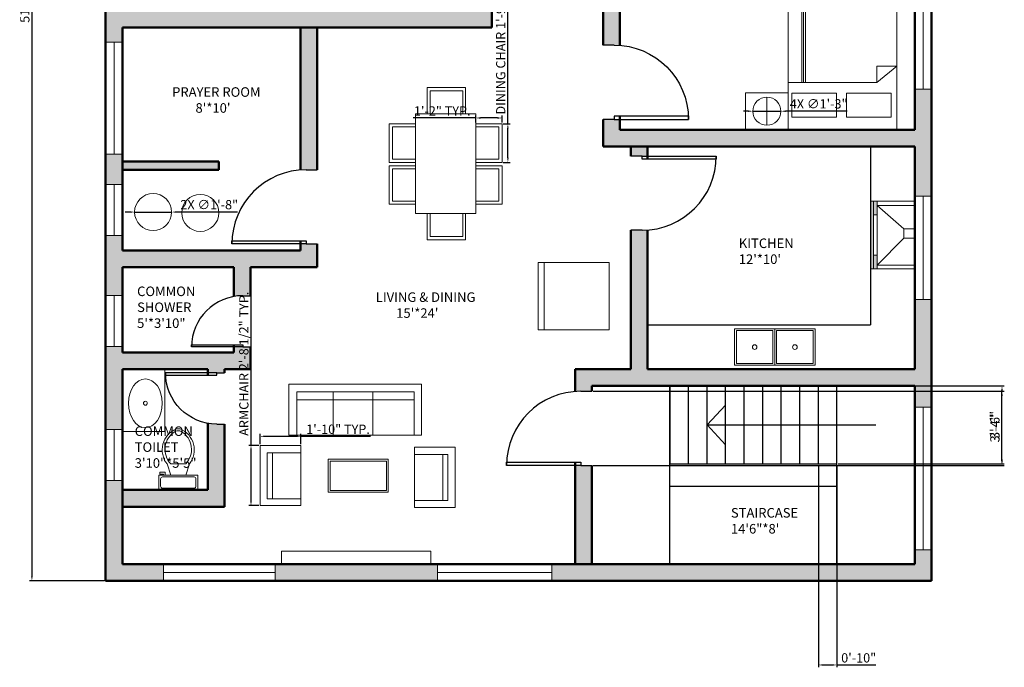
# Model space of a CAD drawing. Units: inches. Extents: x 2091 to 2624, y 1080 to 1790.
# Tile 1 of 2: x 2091 to 2621, y 1080 to 1429. Entities that reach past the tile are written whole.
import ezdxf

# ---------------------------------------------------------------- set-up
doc = ezdxf.new("R2010")
doc.units = ezdxf.units.IN
for name, color, linetype, lineweight in [('A-ANNO-DIMS', 135, 'Continuous', 18), ('A-AREA-IDEN', 135, 'Continuous', 18), ('A-EQPM', 210, 'Continuous', 18), ('A-EQPM-PATT', 210, 'Continuous', 13), ('A-FLOR-CASE', 210, 'Continuous', 25), ('A-FLOR-FIXT', 210, 'Continuous', 18), ('A-FLOR-STRS', 7, 'Continuous', 25), ('A-WALL-PATT', 190, 'Continuous', 13), ('DOOR', 20, 'Continuous', 25), ('FUR', 210, 'Continuous', 18), ('WALL', 190, 'Continuous', 50), ('WIND', 10, 'Continuous', 18)]:
    doc.layers.add(name, color=color, linetype=linetype, lineweight=lineweight)
doc.styles.get("Standard").update_dxf_attribs({"font": 'arial.ttf'})
doc.dimstyles.new('ISO-25', dxfattribs={"dimtxt": 5, "dimasz": 2.5, "dimexe": 1.25, "dimexo": 0.625, "dimtad": 1, "dimdec": 0, "dimlunit": 4, "dimtxsty": 'Standard', "dimcen": 2.5, "dimadec": 0, "dimazin": 0, "dimtfac": 1, "dimtdec": 0, "dimtmove": 0, "dimatfit": 3, "dimfxl": 1, "dimarcsym": 0})

# ---------------------------------------------------------------- blocks, each defined once
blk = doc.blocks.new('*U2')
for p, q in [((0, 0), (0, -6)), ((40, 0), (40, -6))]:
    blk.add_line(p, q)
blk.add_lwpolyline([(0, 0), (0, 40), (1.75, 40), (1.75, 0)], close=True)
blk.add_arc((0, 0), 40, 0, 90)
blk = doc.blocks.new('*U4')
for p, q in [((9.5, -6), (9.5, -2)), ((-10, -8.5), (-8, -8.5)), ((-10, -9.5), (-10, -8.5)), ((-7, -9.5), (-10, -9.5)), ((-8, -8.5), (-8, -8)), ((-7, -8), (-7, -9.5)), ((-4, -8), (-6, -14)), ((4, -8), (6, -14)), ((4, -14), (-4, -14))]:
    blk.add_line(p, q)
blk.add_lwpolyline([(10.5, -8), (10.5, 0), (-10.5, 0), (-10.5, -8)], close=True)
for points in [[(-9.5, -2), (-9.5, -6)], [(8.5, -1), (-8.5, -1)], [(-8.5, -7), (8.5, -7)]]:
    blk.add_lwpolyline(points)
for centre, radius, start, end in [((-8.62, -1.88), 0.884, 81.8699, 188.1301), ((8.62, -1.88), 0.884, 351.8699, 98.1301), ((-8.62, -6.12), 0.884, 171.8699, 278.1301), ((8.62, -6.12), 0.884, 261.8699, 8.1301), ((3.52, -21.58), 12.17, 141.4691, 247.9714), ((4.2, -21.82), 11.33, 136.3677, 238.9468), ((-3.52, -21.58), 12.17, 292.0284, 38.5307), ((-4.2, -21.82), 11.33, 301.053, 43.6321), ((0, -27.88), 4, 245.7318, 294.2682), ((0, -29), 4, 254.8605, 285.1395)]:
    blk.add_arc(centre, radius, start, end)
blk = doc.blocks.new('*D8')
at = {"layer": 'A-ANNO-DIMS', "color": 0, "lineweight": -2, "transparency": 16777216}
for p, q in [((2136.64, 1746.37), (2096.29, 1746.37)), ((2097.54, 1743.87), (2097.54, 1128.87)), ((2136.64, 1126.37), (2096.29, 1126.37))]:
    blk.add_line(p, q, dxfattribs=at)
at = {"layer": 'A-ANNO-DIMS', "color": 0, "transparency": 16777216}
for points in [[(2097.12, 1743.87), (2097.96, 1743.87), (2097.54, 1746.37)], [(2097.12, 1128.87), (2097.96, 1128.87), (2097.54, 1126.37)]]:
    blk.add_solid(points, dxfattribs=at)
at = {"layer": 'Defpoints', "color": 0, "transparency": 16777216}
for p in [(2137.27, 1746.37), (2097.54, 1126.37), (2137.27, 1126.37)]:
    blk.add_point(p, dxfattribs=at)
at = {"layer": 'A-ANNO-DIMS', "color": 0, "transparency": 16777216, "insert": (2094.36, 1436.37), "char_height": 5, "attachment_point": 5, "rotation": 90}
blk.add_mtext('51\'-8"', dxfattribs=at)
blk = doc.blocks.new('ARMCHAIR')
for p, q in [((0, 28.45), (0, 32.47)), ((0, 32.47), (21.94, 32.47)), ((21.94, 32.47), (21.94, 28.45)), ((0, 0), (0, 28.45)), ((6.7, 3.68), (6.7, 28.45)), ((3.85, 0), (0, 0)), ((21.94, 0), (3.85, 0)), ((21.94, 3.68), (21.94, 0))]:
    blk.add_line(p, q)
blk.add_lwpolyline([(21.94, 28.45), (3.85, 28.45), (3.85, 3.68), (21.94, 3.68)], close=True)
blk = doc.blocks.new('DINING-CHAIR')
for p, q in [((0, 14.12), (0, 0)), ((20.77, 0), (20.77, 14.12)), ((0, 0), (20.77, 0))]:
    blk.add_line(p, q)
blk.add_lwpolyline([(1.63, 14.12), (19.2, 14.12), (19.2, 1.73), (1.63, 1.73)], close=True)
blk = doc.blocks.new('BED-DOUBLE')
for p, q in [((7.26, 25.51), (7.26, 77.87)), ((8.26, 25.51), (8.26, 77.87)), ((9.26, 25.51), (9.26, 77.87)), ((0, 69.01), (58.45, 69.01)), ((0, 68.01), (58.45, 68.01)), ((0, 67.01), (58.45, 67.01)), ((47.64, 25.51), (47.64, 34.16)), ((47.64, 34.16), (58.45, 34.16)), ((58.45, 34.16), (47.64, 25.51)), ((0, 25.51), (47.64, 25.51))]:
    blk.add_line(p, q)
for points in [[(0, 0), (58.45, 0), (58.45, 77.87), (0, 77.87)], [(1.98, 6.84), (26.02, 6.84), (26.02, 19.63), (1.98, 19.63)], [(31.32, 6.84), (55.36, 6.84), (55.36, 19.63), (31.32, 19.63)]]:
    blk.add_lwpolyline(points, close=True)
blk = doc.blocks.new('NIGHTSTAND-LAMP')
for p, q in [((11.52, 2.41), (11.52, 17.54)), ((3.95, 9.98), (19.08, 9.98)), ((11.52, 9.98), (11.52, 2.41))]:
    blk.add_line(p, q)
blk.add_lwpolyline([(23.03, 0), (0, 0), (0, 19.96), (23.03, 19.96)], close=True)
blk.add_circle((11.52, 9.98), 7.56)
blk = doc.blocks.new('LAVATORY-BASIN')
blk.add_circle((9.11, 13.13), 1.04)
blk.add_ellipse((9.11, 13.13), major_axis=(0, 13.13), ratio=0.694107)
blk = doc.blocks.new('WIN-76_81')
blk.add_line((0, 4.5), (76.81, 4.5))
blk.add_lwpolyline([(0, 0), (76.81, 0), (76.81, 9), (0, 9)], close=True)
blk = doc.blocks.new('WIN-27_52')
blk.add_line((0, 4.5), (27.52, 4.5))
blk.add_lwpolyline([(0, 0), (27.52, 0), (27.52, 9), (0, 9)], close=True)
blk = doc.blocks.new('*D26')
at = {"layer": 'A-ANNO-DIMS', "color": 0, "lineweight": -2, "transparency": 16777216}
for p, q in [((2353.97, 1372.58), (2353.97, 1456.62)), ((2351.48, 1372.58), (2355.22, 1372.58)), ((2353.97, 1354.31), (2353.97, 1370.08)), ((2351.48, 1351.81), (2355.22, 1351.81))]:
    blk.add_line(p, q, dxfattribs=at)
at = {"layer": 'A-ANNO-DIMS', "color": 0, "transparency": 16777216}
for points in [[(2353.56, 1370.08), (2354.39, 1370.08), (2353.97, 1372.58)], [(2353.56, 1354.31), (2354.39, 1354.31), (2353.97, 1351.81)]]:
    blk.add_solid(points, dxfattribs=at)
at = {"layer": 'Defpoints', "color": 0, "transparency": 16777216}
for p in [(2350.86, 1372.58), (2353.97, 1372.58), (2350.86, 1351.81)]:
    blk.add_point(p, dxfattribs=at)
at = {"layer": 'A-ANNO-DIMS', "color": 0, "transparency": 16777216, "insert": (2350.76, 1415.85), "char_height": 5, "attachment_point": 5, "rotation": 90}
blk.add_mtext('DINING CHAIR 1\'-9" TYP.', dxfattribs=at)
blk = doc.blocks.new('*D27')
at = {"layer": 'A-ANNO-DIMS', "color": 0, "lineweight": -2, "transparency": 16777216}
for p, q in [((2336.74, 1375.7), (2302.99, 1375.7)), ((2336.74, 1373.2), (2336.74, 1376.95)), ((2348.36, 1375.7), (2339.24, 1375.7)), ((2350.86, 1373.2), (2350.86, 1376.95))]:
    blk.add_line(p, q, dxfattribs=at)
at = {"layer": 'A-ANNO-DIMS', "color": 0, "transparency": 16777216}
for points in [[(2339.24, 1376.11), (2339.24, 1375.28), (2336.74, 1375.7)], [(2348.36, 1376.11), (2348.36, 1375.28), (2350.86, 1375.7)]]:
    blk.add_solid(points, dxfattribs=at)
at = {"layer": 'Defpoints', "color": 0, "transparency": 16777216}
for p in [(2336.74, 1375.7), (2336.74, 1372.58), (2350.86, 1372.58)]:
    blk.add_point(p, dxfattribs=at)
at = {"layer": 'A-ANNO-DIMS', "color": 0, "transparency": 16777216, "insert": (2318.61, 1378.83), "char_height": 5, "attachment_point": 5}
blk.add_mtext('1\'-2" TYP.', dxfattribs=at)
blk = doc.blocks.new('*D28')
at = {"layer": 'A-ANNO-DIMS', "color": 0, "lineweight": -2, "transparency": 16777216}
for p, q in [((2215.58, 1199.39), (2215.58, 1284.76)), ((2219.82, 1199.39), (2214.33, 1199.39)), ((2215.58, 1169.43), (2215.58, 1196.89)), ((2219.82, 1166.93), (2214.33, 1166.93))]:
    blk.add_line(p, q, dxfattribs=at)
at = {"layer": 'A-ANNO-DIMS', "color": 0, "transparency": 16777216}
for points in [[(2215.16, 1196.89), (2215.99, 1196.89), (2215.58, 1199.39)], [(2215.16, 1169.43), (2215.99, 1169.43), (2215.58, 1166.93)]]:
    blk.add_solid(points, dxfattribs=at)
at = {"layer": 'Defpoints', "color": 0, "transparency": 16777216}
for p in [(2215.58, 1199.39), (2220.45, 1199.39), (2220.45, 1166.93)]:
    blk.add_point(p, dxfattribs=at)
at = {"layer": 'A-ANNO-DIMS', "color": 0, "transparency": 16777216, "insert": (2212.37, 1243.33), "char_height": 5, "attachment_point": 5, "rotation": 90}
blk.add_mtext('ARMCHAIR 2\'-8 1/2" TYP.', dxfattribs=at)
blk = doc.blocks.new('*D29')
at = {"layer": 'A-ANNO-DIMS', "color": 0, "lineweight": -2, "transparency": 16777216}
for p, q in [((2220.45, 1200.02), (2220.45, 1205.51)), ((2222.95, 1204.26), (2239.89, 1204.26)), ((2242.39, 1200.02), (2242.39, 1205.51)), ((2242.39, 1204.26), (2280.03, 1204.26))]:
    blk.add_line(p, q, dxfattribs=at)
at = {"layer": 'A-ANNO-DIMS', "color": 0, "transparency": 16777216}
for points in [[(2222.95, 1204.68), (2222.95, 1203.85), (2220.45, 1204.26)], [(2239.89, 1204.68), (2239.89, 1203.85), (2242.39, 1204.26)]]:
    blk.add_solid(points, dxfattribs=at)
at = {"layer": 'Defpoints', "color": 0, "transparency": 16777216}
for p in [(2242.39, 1204.26), (2220.45, 1199.39), (2242.39, 1199.39)]:
    blk.add_point(p, dxfattribs=at)
at = {"layer": 'A-ANNO-DIMS', "color": 0, "transparency": 16777216, "insert": (2262.46, 1207.44), "char_height": 5, "attachment_point": 5}
blk.add_mtext('1\'-10" TYP.', dxfattribs=at)
blk = doc.blocks.new('*D30')
at = {"layer": 'A-ANNO-DIMS', "color": 0, "lineweight": -2, "transparency": 16777216}
for p, q in [((2399.89, 1228.51), (2621.44, 1228.51)), ((2620.19, 1191.01), (2620.19, 1226.01)), ((2399.89, 1188.51), (2621.44, 1188.51))]:
    blk.add_line(p, q, dxfattribs=at)
at = {"layer": 'A-ANNO-DIMS', "color": 0, "transparency": 16777216}
for points in [[(2619.77, 1226.01), (2620.6, 1226.01), (2620.19, 1228.51)], [(2619.77, 1191.01), (2620.6, 1191.01), (2620.19, 1188.51)]]:
    blk.add_solid(points, dxfattribs=at)
at = {"layer": 'Defpoints', "color": 0, "transparency": 16777216}
for p in [(2399.27, 1228.51), (2620.19, 1228.51), (2399.27, 1188.51)]:
    blk.add_point(p, dxfattribs=at)
at = {"layer": 'A-ANNO-DIMS', "color": 0, "transparency": 16777216, "insert": (2617.01, 1208.51), "char_height": 5, "attachment_point": 5, "rotation": 90}
blk.add_mtext('3\'-4"', dxfattribs=at)
blk = doc.blocks.new('*D32')
at = {"layer": 'A-ANNO-DIMS', "color": 0, "lineweight": -2, "transparency": 16777216}
for p, q in [((2531.89, 1231.37), (2621.44, 1231.37)), ((2620.19, 1191.87), (2620.19, 1228.87)), ((2531.89, 1189.37), (2621.44, 1189.37))]:
    blk.add_line(p, q, dxfattribs=at)
at = {"layer": 'A-ANNO-DIMS', "color": 0, "transparency": 16777216}
for points in [[(2619.77, 1228.87), (2620.6, 1228.87), (2620.19, 1231.37)], [(2619.77, 1191.87), (2620.6, 1191.87), (2620.19, 1189.37)]]:
    blk.add_solid(points, dxfattribs=at)
at = {"layer": 'Defpoints', "color": 0, "transparency": 16777216}
for p in [(2531.27, 1231.37), (2620.19, 1231.37), (2531.27, 1189.37)]:
    blk.add_point(p, dxfattribs=at)
at = {"layer": 'A-ANNO-DIMS', "color": 0, "transparency": 16777216, "insert": (2617.01, 1210.37), "char_height": 5, "attachment_point": 5, "rotation": 90}
blk.add_mtext('3\'-6"', dxfattribs=at)
blk = doc.blocks.new('*D33')
at = {"layer": 'A-ANNO-DIMS', "color": 0, "lineweight": -2, "transparency": 16777216}
for p, q in [((2521.27, 1188.74), (2521.27, 1079.87)), ((2531.27, 1188.74), (2531.27, 1079.87)), ((2523.77, 1081.12), (2528.77, 1081.12)), ((2531.27, 1081.12), (2552.19, 1081.12))]:
    blk.add_line(p, q, dxfattribs=at)
at = {"layer": 'A-ANNO-DIMS', "color": 0, "transparency": 16777216}
for points in [[(2523.77, 1081.53), (2523.77, 1080.7), (2521.27, 1081.12)], [(2528.77, 1081.53), (2528.77, 1080.7), (2531.27, 1081.12)]]:
    blk.add_solid(points, dxfattribs=at)
at = {"layer": 'Defpoints', "color": 0, "transparency": 16777216}
for p in [(2521.27, 1189.37), (2531.27, 1189.37), (2531.27, 1081.12)]:
    blk.add_point(p, dxfattribs=at)
at = {"layer": 'A-ANNO-DIMS', "color": 0, "transparency": 16777216, "insert": (2542.98, 1084.29), "char_height": 5, "attachment_point": 5}
blk.add_mtext('0\'-10"', dxfattribs=at)
blk = doc.blocks.new('*D34')
at = {"layer": 'A-ANNO-DIMS', "color": 0, "lineweight": -2, "transparency": 16777216}
for p, q in [((2150.37, 1325.04), (2147.87, 1325.04)), ((2152.87, 1325.04), (2172.8, 1325.04)), ((2208.34, 1325.04), (2175.3, 1325.04))]:
    blk.add_line(p, q, dxfattribs=at)
at = {"layer": 'A-ANNO-DIMS', "color": 0, "transparency": 16777216}
for points in [[(2150.37, 1325.46), (2150.37, 1324.62), (2152.87, 1325.04)], [(2175.3, 1325.46), (2175.3, 1324.62), (2172.8, 1325.04)]]:
    blk.add_solid(points, dxfattribs=at)
at = {"layer": 'Defpoints', "color": 0, "transparency": 16777216}
for p in [(2152.87, 1325.04), (2172.8, 1325.04)]:
    blk.add_point(p, dxfattribs=at)
at = {"layer": 'A-ANNO-DIMS', "color": 0, "transparency": 16777216, "insert": (2193.07, 1328.36), "char_height": 5, "attachment_point": 5, "rotation": 359.9978}
blk.add_mtext('2X ∅1\'-8"', dxfattribs=at)
blk = doc.blocks.new('*D35')
at = {"layer": 'A-ANNO-DIMS', "color": 0, "lineweight": -2, "transparency": 16777216}
for p, q in [((2483.46, 1379.35), (2480.96, 1379.35)), ((2485.96, 1379.35), (2501.09, 1379.35)), ((2536.75, 1379.35), (2503.59, 1379.35))]:
    blk.add_line(p, q, dxfattribs=at)
at = {"layer": 'A-ANNO-DIMS', "color": 0, "transparency": 16777216}
for points in [[(2483.46, 1379.76), (2483.46, 1378.93), (2485.96, 1379.35)], [(2503.59, 1379.76), (2503.59, 1378.93), (2501.09, 1379.35)]]:
    blk.add_solid(points, dxfattribs=at)
at = {"layer": 'Defpoints', "color": 0, "transparency": 16777216}
for p in [(2485.96, 1379.35), (2501.09, 1379.35)]:
    blk.add_point(p, dxfattribs=at)
at = {"layer": 'A-ANNO-DIMS', "color": 0, "transparency": 16777216, "insert": (2521.42, 1382.66), "char_height": 5, "attachment_point": 5, "rotation": 0.0023}
blk.add_mtext('4X ∅1\'-3"', dxfattribs=at)

msp = doc.modelspace()

# ---------------------------------------------------------------- hatches: boundary and pattern name
at = {"layer": 'A-EQPM-PATT'}
h = msp.add_hatch(color=256, dxfattribs=at)
h.dxf.hatch_style = 1
h.paths.add_polyline_path([(2553.02, 1330.86), (2550.94, 1330.86), (2550.94, 1323.49), (2553.02, 1323.49)])
h.paths.add_polyline_path([(2553.02, 1301.86), (2550.94, 1301.86), (2550.94, 1294.49), (2553.02, 1294.49)])
h.paths.add_polyline_path([(2550.94, 1330.86), (2549.27, 1330.86), (2549.27, 1294.49), (2550.94, 1294.49), (2550.94, 1301.86)])
at = {"layer": 'A-WALL-PATT'}
h = msp.add_hatch(color=256, dxfattribs=at)
h.dxf.hatch_style = 1
h.paths.add_polyline_path([(2203.27, 1737.37), (2203.27, 1746.37), (2194.27, 1746.37), (2194.27, 1703.2, -0.044322), (2199.13, 1703.63), (2203.27, 1703.63)])
h.paths.add_polyline_path([(2238.46, 1746.37), (2203.27, 1746.37), (2203.27, 1737.37), (2238.46, 1737.37)])
h.paths.add_polyline_path([(2194.27, 1593.37), (2146.27, 1593.37), (2146.27, 1596.35), (2137.27, 1596.35), (2137.27, 1584.37), (2194.27, 1584.37)])
h.paths.add_polyline_path([(2146.27, 1584.37), (2137.27, 1584.37), (2137.27, 1548.65), (2146.27, 1548.65)])
h.paths.add_polyline_path([(2203.27, 1554.64), (2199.13, 1554.64, -0.044322), (2194.27, 1555.07), (2194.27, 1516.37), (2146.27, 1516.37), (2146.27, 1521.14), (2137.27, 1521.14), (2137.27, 1507.37), (2203.27, 1507.37)])
h.paths.add_polyline_path([(2345.27, 1436.81), (2339.27, 1436.81), (2336.27, 1436.81), (2336.27, 1433.37), (2203.27, 1433.37), (2203.27, 1453.32), (2203.27, 1477.02), (2199.13, 1477.02, -0.044322), (2194.27, 1477.45), (2194.27, 1433.37), (2137.27, 1433.37), (2137.27, 1424.37), (2137.27, 1416.56), (2146.27, 1416.56), (2146.27, 1424.37), (2242.27, 1424.37), (2345.27, 1424.37)])
h.paths.add_polyline_path([(2345.27, 1557.08), (2336.27, 1557.08), (2336.27, 1512.08), (2336.27, 1476.7, -0.01877), (2339.27, 1476.81), (2345.27, 1476.81)])
h.paths.add_polyline_path([(2146.27, 1356.3), (2137.27, 1356.3), (2137.27, 1339.9), (2146.27, 1339.9)])
h.paths.add_polyline_path([(2251.27, 1307.84), (2245.27, 1307.84), (2242.27, 1307.84), (2242.27, 1304.37), (2146.27, 1304.37), (2146.27, 1312.38), (2137.27, 1312.38), (2137.27, 1295.37), (2137.27, 1280.09), (2146.27, 1280.09), (2146.27, 1295.37), (2206.27, 1295.37), (2206.27, 1279.55, -0.044322), (2211.13, 1279.98), (2215.27, 1279.98), (2215.27, 1295.37), (2251.27, 1295.37)])
h.paths.add_polyline_path([(2251.27, 1424.37), (2242.27, 1424.37), (2242.27, 1347.73, -0.01877), (2245.27, 1347.84), (2251.27, 1347.84)])
h.paths.add_polyline_path([(2146.27, 1240.37), (2169.1, 1240.37), (2192.27, 1240.37), (2192.27, 1238.44), (2197.13, 1238.44), (2201.27, 1238.44), (2201.27, 1240.37), (2215.27, 1240.37), (2215.27, 1252.39), (2211.13, 1252.39), (2206.27, 1252.39), (2206.27, 1249.37), (2146.27, 1249.37), (2146.27, 1252.57), (2137.27, 1252.57), (2137.27, 1240.37), (2137.27, 1208.01), (2146.27, 1208.01)])
h.paths.add_polyline_path([(2146.27, 1180.49), (2137.27, 1180.49), (2137.27, 1126.37), (2168.5, 1126.37), (2168.5, 1135.37), (2146.27, 1135.37)])
h.paths.add_polyline_path([(2316.01, 1135.37), (2228.53, 1135.37), (2228.53, 1126.37), (2316.01, 1126.37)])
h.paths.add_polyline_path([(2582.27, 1143.15), (2573.27, 1143.15), (2573.27, 1135.37), (2531.27, 1135.37), (2377.62, 1135.37), (2377.62, 1126.37), (2582.27, 1126.37)])
h.paths.add_polyline_path([(2582.27, 1277.86), (2573.27, 1277.86), (2573.27, 1240.37), (2429.27, 1240.37), (2429.27, 1264.37), (2429.27, 1315.33, -0.01877), (2426.27, 1315.22), (2420.27, 1315.22), (2420.27, 1240.37), (2390.27, 1240.37), (2390.27, 1228.4, -0.01877), (2393.27, 1228.51), (2399.27, 1228.51), (2399.27, 1231.37), (2420.27, 1231.37), (2573.27, 1231.37), (2573.27, 1219.96), (2582.27, 1219.96), (2582.27, 1231.37)])
h.paths.add_polyline_path([(2582.27, 1391.21), (2573.27, 1391.21), (2573.27, 1369.37), (2414.27, 1369.37), (2414.27, 1374.96), (2411.27, 1374.96), (2405.27, 1374.96), (2405.27, 1360.37), (2573.27, 1360.37), (2573.27, 1333.61), (2582.27, 1333.61), (2582.27, 1360.37)])
h.paths.add_polyline_path([(2582.27, 1541.89), (2573.27, 1541.89), (2573.27, 1509.37), (2414.27, 1509.37), (2414.27, 1514.26), (2411.27, 1514.26), (2405.27, 1514.26), (2405.27, 1500.37), (2405.27, 1414.96), (2411.27, 1414.96, -0.01877), (2414.27, 1414.85), (2414.27, 1500.37), (2477.45, 1500.37), (2573.27, 1500.37), (2573.27, 1468.02), (2582.27, 1468.02), (2582.27, 1500.37)])
h.paths.add_polyline_path([(2236.44, 1532.62), (2267.09, 1532.62), (2267.09, 1551.82), (2236.44, 1551.82)], flags=9)
h.paths.add_polyline_path([(2148.33, 1605.52), (2176.06, 1605.52), (2176.06, 1624.71), (2148.33, 1624.71)], flags=9)
h.paths.add_polyline_path([(2360.41, 1679.17), (2404.5, 1679.17), (2404.5, 1698.37), (2360.41, 1698.37)], flags=9)
h.paths.add_polyline_path([(2484.05, 1685.08), (2521.22, 1685.08), (2521.22, 1704.27), (2484.05, 1704.27)], flags=9)
h.paths.add_polyline_path([(2450.18, 1596.03), (2522.07, 1596.03), (2522.07, 1615.22), (2450.18, 1615.22)], flags=9)
h.paths.add_polyline_path([(2482.78, 1454.78), (2549.63, 1454.78), (2549.63, 1473.97), (2482.78, 1473.97)], flags=25)
h.paths.add_polyline_path([(2476.32, 1294.17), (2510.69, 1294.17), (2510.69, 1313.36), (2476.32, 1313.36)], flags=25)
h.paths.add_polyline_path([(2281, 1265.16), (2341.07, 1265.16), (2341.07, 1284.35), (2281, 1284.35)], flags=9)
h.paths.add_polyline_path([(2151.29, 1184.31), (2187.39, 1184.31), (2187.39, 1212.17), (2151.29, 1212.17)], flags=9)
h.paths.add_polyline_path([(2152.56, 1259.62), (2188.66, 1259.62), (2188.66, 1287.47), (2152.56, 1287.47)], flags=9)
h.paths.add_polyline_path([(2171.26, 1375.61), (2227.73, 1375.61), (2227.73, 1394.8), (2171.26, 1394.8)], flags=9)
h.paths.add_polyline_path([(2145.13, 1464.78), (2182.05, 1464.78), (2182.05, 1483.97), (2145.13, 1483.97)], flags=9)
h.paths.add_polyline_path([(2147.67, 1525.88), (2175.4, 1525.88), (2175.4, 1545.07), (2147.67, 1545.07)], flags=25)
h.paths.add_polyline_path([(2237.82, 1687.57), (2268.47, 1687.57), (2268.47, 1706.76), (2237.82, 1706.76)], flags=9)
h.paths.add_polyline_path([(2141.34, 1688.84), (2178.25, 1688.84), (2178.25, 1708.04), (2141.34, 1708.04)], flags=9)
h = msp.add_hatch(color=256, dxfattribs=at)
h.dxf.hatch_style = 1
h.paths.add_polyline_path([(2399.27, 1188.51), (2393.27, 1188.51), (2390.27, 1188.51), (2390.27, 1135.37), (2399.27, 1135.37)])
h.paths.add_polyline_path([(2429.27, 1360.37), (2420.27, 1360.37), (2420.27, 1355.22), (2426.27, 1355.22), (2429.27, 1355.22)])
h.paths.add_polyline_path([(2198.16, 1352.23), (2184.99, 1352.23), (2146.27, 1352.23), (2146.27, 1347.73), (2184.99, 1347.73), (2198.16, 1347.73)])
h.paths.add_polyline_path([(2203.27, 1507.37), (2194.27, 1507.37), (2194.27, 1504.61), (2199.13, 1504.61), (2203.27, 1504.61)])
h = msp.add_hatch(color=256, dxfattribs=at)
h.dxf.hatch_style = 1
h.paths.add_polyline_path([(2201.27, 1210.86), (2197.13, 1210.86, -0.044322), (2192.27, 1211.29), (2192.27, 1175.37), (2146.27, 1175.37), (2146.27, 1166.37), (2201.27, 1166.37)])

# ---------------------------------------------------------------- linework, layer by layer
at = {"layer": 'A-EQPM'}
for p, q in [((2550.94, 1294.49), (2550.94, 1330.86)), ((2553.02, 1294.49), (2553.02, 1330.86)), ((2553.02, 1328.54), (2573.27, 1328.54)), ((2567.36, 1315.93), (2553.02, 1328.54)), ((2567.36, 1310.91), (2553.02, 1296.46)), ((2553.02, 1296.46), (2573.27, 1296.46))]:
    msp.add_line(p, q, dxfattribs=at)
for points in [[(2573.27, 1330.86), (2549.27, 1330.86), (2549.27, 1294.49), (2573.27, 1294.49)], [(2550.94, 1330.86), (2553.02, 1330.86), (2553.02, 1323.49), (2550.94, 1323.49)], [(2573.27, 1315.93), (2567.36, 1315.93), (2567.36, 1310.91), (2573.27, 1310.91)], [(2550.94, 1301.86), (2553.02, 1301.86), (2553.02, 1294.49), (2550.94, 1294.49)]]:
    msp.add_lwpolyline(points, close=True, dxfattribs=at)
at = {"layer": 'A-FLOR-CASE'}
for p, q in [((2573.27, 1360.37), (2549.27, 1360.37)), ((2549.27, 1360.37), (2549.27, 1264.37)), ((2429.27, 1240.37), (2429.27, 1264.37)), ((2429.27, 1264.37), (2549.27, 1264.37))]:
    msp.add_line(p, q, dxfattribs=at)
at = {"layer": 'A-FLOR-FIXT'}
msp.add_line((2497.77, 1242.5), (2497.77, 1262.19), dxfattribs=at)
for points in [[(2476.1, 1262.19), (2519.45, 1262.19), (2519.45, 1242.5), (2476.1, 1242.5)], [(2476.1, 1262.19), (2497.77, 1262.19), (2497.77, 1242.5), (2476.1, 1242.5)], [(2477.1, 1261.19), (2496.77, 1261.19), (2496.77, 1243.5), (2477.1, 1243.5)], [(2497.77, 1242.5), (2519.45, 1242.5), (2519.45, 1262.19), (2497.77, 1262.19)], [(2498.77, 1243.5), (2518.45, 1243.5), (2518.45, 1261.19), (2498.77, 1261.19)], [(2146.27, 1206.79), (2169.1, 1206.79), (2169.1, 1240.37), (2146.27, 1240.37)]]:
    msp.add_lwpolyline(points, close=True, dxfattribs=at)
for centre in [(2486.93, 1252.34), (2508.61, 1252.34)]:
    msp.add_circle(centre, 1.24, dxfattribs=at)
at = {"layer": 'A-FLOR-STRS'}
for p, q in [((2441.27, 1135.37), (2441.27, 1231.37)), ((2441.27, 1231.37), (2441.27, 1189.37)), ((2451.27, 1189.37), (2451.27, 1231.37)), ((2461.27, 1189.37), (2461.27, 1231.37)), ((2471.27, 1189.37), (2471.27, 1231.37)), ((2481.27, 1189.37), (2481.27, 1231.37)), ((2491.27, 1189.37), (2491.27, 1231.37)), ((2501.27, 1189.37), (2501.27, 1231.37)), ((2511.27, 1189.37), (2511.27, 1231.37)), ((2521.27, 1189.37), (2521.27, 1231.37)), ((2531.27, 1135.37), (2531.27, 1231.37)), ((2531.27, 1189.37), (2531.27, 1231.37)), ((2461.27, 1210.37), (2471.27, 1221.12)), ((2461.27, 1210.37), (2552.15, 1210.37)), ((2461.27, 1210.37), (2471.27, 1199.61)), ((2441.27, 1189.37), (2531.27, 1189.37)), ((2441.27, 1135.37), (2441.27, 1177.37)), ((2441.27, 1177.37), (2531.27, 1177.37)), ((2399.27, 1135.37), (2441.27, 1135.37)), ((2573.27, 1135.37), (2531.27, 1135.37))]:
    msp.add_line(p, q, dxfattribs=at)
at = {"layer": 'FUR'}
for p, q in [((2310.44, 1377.97), (2310.44, 1392.09)), ((2310.44, 1392.09), (2331.22, 1392.09)), ((2331.22, 1392.09), (2331.22, 1377.97)), ((2312.08, 1377.97), (2310.44, 1377.97)), ((2373.53, 1261.63), (2373.53, 1297.86)), ((2235.99, 1228.15), (2235.99, 1232.28)), ((2235.99, 1232.28), (2303.55, 1232.28)), ((2303.55, 1232.28), (2307.49, 1232.28)), ((2307.49, 1232.28), (2307.49, 1204.94)), ((2235.99, 1204.94), (2235.99, 1228.15)), ((2259.77, 1228.15), (2259.77, 1204.94)), ((2281.22, 1228.15), (2281.22, 1204.94)), ((2240.2, 1223.97), (2303.55, 1223.97)), ((2240.2, 1204.94), (2235.99, 1204.94)), ((2307.49, 1204.94), (2303.55, 1204.94))]:
    msp.add_line(p, q, dxfattribs=at)
for points in [[(2312.08, 1377.97), (2329.64, 1377.97), (2329.64, 1390.35), (2312.08, 1390.35)], [(2304.2, 1324.26), (2336.74, 1324.26), (2336.74, 1377.97), (2304.2, 1377.97)], [(2408.58, 1261.63), (2370.37, 1261.63), (2370.37, 1297.86), (2408.58, 1297.86)], [(2240.2, 1228.15), (2303.55, 1228.15), (2303.55, 1204.94), (2240.2, 1204.94)], [(2257.22, 1191.89), (2289.56, 1191.89), (2289.56, 1174.12), (2257.22, 1174.12)], [(2258.22, 1190.89), (2288.56, 1190.89), (2288.56, 1175.12), (2258.22, 1175.12)], [(2231.94, 1135.37), (2312.47, 1135.37), (2312.47, 1142.33), (2231.94, 1142.33)]]:
    msp.add_lwpolyline(points, close=True, dxfattribs=at)
for centre in [(2162.83, 1325.04), (2188.26, 1324.6)]:
    msp.add_circle(centre, 9.97, dxfattribs=at)
at = {"layer": 'WALL'}
for p, q in [((2137.27, 1424.37), (2137.27, 1517.37)), ((2405.27, 1500.37), (2405.27, 1414.96)), ((2414.27, 1500.37), (2414.27, 1414.85)), ((2573.27, 1500.37), (2573.27, 1369.37)), ((2582.27, 1500.37), (2582.27, 1360.37)), ((2345.27, 1424.37), (2345.27, 1436.81)), ((2137.27, 1424.37), (2137.27, 1295.37)), ((2203.27, 1424.37), (2146.27, 1424.37)), ((2146.27, 1424.37), (2146.27, 1304.37)), ((2146.27, 1424.37), (2242.27, 1424.37)), ((2203.27, 1424.37), (2345.27, 1424.37)), ((2242.27, 1424.37), (2242.27, 1347.73)), ((2251.27, 1424.37), (2251.27, 1347.84)), ((2405.27, 1374.96), (2405.27, 1360.37)), ((2414.27, 1376.71), (2414.27, 1369.37)), ((2414.27, 1369.37), (2573.27, 1369.37)), ((2405.27, 1360.37), (2573.27, 1360.37)), ((2420.27, 1360.37), (2420.27, 1355.22)), ((2573.27, 1360.37), (2429.27, 1360.37)), ((2429.27, 1360.37), (2429.27, 1353.47)), ((2573.27, 1360.37), (2573.27, 1240.37)), ((2582.27, 1360.37), (2582.27, 1231.37)), ((2184.99, 1352.23), (2146.27, 1352.23)), ((2184.99, 1347.73), (2146.27, 1347.73)), ((2184.99, 1352.23), (2198.16, 1352.23)), ((2184.99, 1347.73), (2198.16, 1347.73)), ((2198.16, 1347.73), (2198.16, 1352.23)), ((2420.27, 1315.22), (2420.27, 1240.37)), ((2429.27, 1315.33), (2429.27, 1240.37)), ((2242.27, 1309.59), (2242.27, 1304.37)), ((2251.27, 1307.84), (2251.27, 1295.37)), ((2146.27, 1304.37), (2242.27, 1304.37)), ((2137.27, 1295.37), (2137.27, 1240.37)), ((2146.27, 1295.37), (2206.27, 1295.37)), ((2146.27, 1295.37), (2146.27, 1249.37)), ((2146.27, 1295.37), (2206.27, 1295.37)), ((2206.27, 1295.37), (2206.27, 1279.55)), ((2215.27, 1295.37), (2215.27, 1279.98)), ((2215.27, 1295.37), (2251.27, 1295.37)), ((2206.27, 1253.6), (2206.27, 1249.37)), ((2215.27, 1252.39), (2215.27, 1240.37)), ((2146.27, 1249.37), (2206.27, 1249.37)), ((2137.27, 1240.37), (2137.27, 1126.37)), ((2146.27, 1240.37), (2192.27, 1240.37)), ((2146.27, 1240.37), (2146.27, 1135.37)), ((2146.27, 1240.37), (2192.27, 1240.37)), ((2192.27, 1240.37), (2192.27, 1237.24)), ((2201.27, 1240.37), (2201.27, 1238.44)), ((2201.27, 1240.37), (2215.27, 1240.37)), ((2390.27, 1240.37), (2420.27, 1240.37)), ((2390.27, 1228.4), (2390.27, 1240.37)), ((2429.27, 1240.37), (2573.27, 1240.37)), ((2399.27, 1231.37), (2420.27, 1231.37)), ((2399.27, 1228.51), (2399.27, 1231.37)), ((2420.27, 1231.37), (2573.27, 1231.37)), ((2573.27, 1231.37), (2573.27, 1135.37)), ((2582.27, 1231.37), (2582.27, 1126.37)), ((2192.27, 1211.29), (2192.27, 1175.37)), ((2201.27, 1210.86), (2201.27, 1166.37)), ((2390.27, 1135.37), (2390.27, 1190.26)), ((2399.27, 1135.37), (2399.27, 1188.51)), ((2192.27, 1175.37), (2146.27, 1175.37)), ((2201.27, 1166.37), (2146.27, 1166.37)), ((2573.27, 1135.37), (2146.27, 1135.37)), ((2582.27, 1126.37), (2137.27, 1126.37))]:
    msp.add_line(p, q, dxfattribs=at)
at = {"layer": 'WIND'}
for p, q in [((2141.77, 1356.3), (2141.77, 1416.56)), ((2577.77, 1277.86), (2577.77, 1333.61)), ((2168.5, 1130.87), (2228.53, 1130.87)), ((2316.01, 1130.87), (2377.62, 1130.87))]:
    msp.add_line(p, q, dxfattribs=at)
for points in [[(2137.27, 1356.3), (2146.27, 1356.3), (2146.27, 1416.56), (2137.27, 1416.56)], [(2573.27, 1333.61), (2582.27, 1333.61), (2582.27, 1277.86), (2573.27, 1277.86)], [(2168.5, 1126.37), (2228.53, 1126.37), (2228.53, 1135.37), (2168.5, 1135.37)], [(2316.01, 1126.37), (2377.62, 1126.37), (2377.62, 1135.37), (2316.01, 1135.37)]]:
    msp.add_lwpolyline(points, close=True, dxfattribs=at)

# ---------------------------------------------------------------- block references
at = {"layer": 'A-FLOR-FIXT'}
msp.add_blockref('LAVATORY-BASIN', (2149.57, 1208.95), dxfattribs=at)
at = {"layer": 'A-FLOR-FIXT', "xscale": -1, "rotation": 180}
msp.add_blockref('*U4', (2176.38, 1175.37), dxfattribs=at)
at = {"layer": 'DOOR', "xscale": -1, "rotation": 270}
msp.add_blockref('*U2', (2411.27, 1374.96), dxfattribs=at)
at = {"layer": 'DOOR'}
for p, rotation in [((2426.27, 1355.22), 270), ((2245.27, 1307.84), 90), ((2393.27, 1188.51), 90)]:
    msp.add_blockref('*U2', p, dxfattribs=dict(at, rotation=rotation))
at = {"layer": 'DOOR', "yscale": 0.689663564140265, "zscale": 0.689663564140265}
for p, xscale, rotation in [((2211.13, 1252.39), 0.689663564140265, 90.00000000000003), ((2197.13, 1238.44), -0.689663564140265, 90)]:
    msp.add_blockref('*U2', p, dxfattribs=dict(at, xscale=xscale, rotation=rotation))
at = {"layer": 'FUR'}
for name, p in [('BED-DOUBLE', (2505.04, 1369.37)), ('NIGHTSTAND-LAMP', (2482.01, 1369.37)), ('DINING-CHAIR', (2310.44, 1310.15)), ('ARMCHAIR', (2220.45, 1166.93))]:
    msp.add_blockref(name, p, dxfattribs=at)
at = {"layer": 'FUR', "extrusion": (0, 0, -1), "zscale": -1}
for p, rotation in [((-2290.08, 1351.81), 90.0000000000019), ((-2290.08, 1329.2), 90.00000000000136)]:
    msp.add_blockref('DINING-CHAIR', p, dxfattribs=dict(at, rotation=rotation))
at = {"layer": 'FUR'}
for p, rotation in [((2350.86, 1351.81), 90.00000000000351), ((2350.86, 1329.2), 90.000000000003)]:
    msp.add_blockref('DINING-CHAIR', p, dxfattribs=dict(at, rotation=rotation))
at = {"layer": 'FUR', "extrusion": (0, 0, -1), "zscale": -1}
msp.add_blockref('ARMCHAIR', (-2325.55, 1165.95), dxfattribs=at)
at = {"layer": 'WIND'}
for name, p, rotation in [('WIN-76_81', (2573.27, 1468.02), 270.0000000000009), ('WIN-27_52', (2137.27, 1339.9), 270.0000000000007), ('WIN-27_52', (2137.27, 1280.09), 270.0000000000002), ('WIN-76_81', (2573.27, 1219.96), 270.0000000000009), ('WIN-27_52', (2137.27, 1208.01), 270.000000000001)]:
    msp.add_blockref(name, p, dxfattribs=dict(at, rotation=rotation))

# ---------------------------------------------------------------- texts
at = {"layer": 'A-AREA-IDEN', "attachment_point": 1}
for s, insert, char_height in [("PRAYER ROOM\\P        8'*10'", (2173.1, 1392.25), 5.1437), ("KITCHEN\\P12'*10'", (2478.39, 1310.8), 5.144), ('COMMON\\PSHOWER\\P5\'*3\'10"', (2154.21, 1284.92), 5.144), ("LIVING & DINING\\P       15'*24'", (2282.81, 1281.79), 5.1437), ('COMMON\\PTOILET\\P3\'10"*5\'5"', (2152.93, 1209.61), 5.144), ('STAIRCASE\\P14\'6"*8\'', (2474.15, 1165.63), 5.144)]:
    msp.add_mtext_dynamic_manual_height_columns(s, width=77.3161, gutter_width=25.72, heights=[0], dxfattribs=dict(at, insert=insert, char_height=char_height))

# ---------------------------------------------------------------- dimensions: what is measured, and where the dimension line sits
at = {"layer": 'A-ANNO-DIMS'}
for base, p1, p2, override, picture, middle in [((2097.54, 1126.37), (2137.27, 1746.37), (2137.27, 1126.37), {"dimclrd": 0, "dimclre": 0, "dimclrt": 0}, '*D8', (2094.36, 1436.37)), ((2620.19, 1231.37), (2531.27, 1189.37), (2531.27, 1231.37), {"dimdec": 1, "dimlfac": 1, "dimrnd": 0, "dimzin": 1, "dimdsep": 46, "dimlunit": 4, "dimfrac": 2}, '*D32', (2617.01, 1210.37)), ((2620.19, 1228.51), (2399.27, 1188.51), (2399.27, 1228.51), {"dimdec": 1, "dimlfac": 1, "dimrnd": 0, "dimzin": 1, "dimdsep": 46, "dimlunit": 4, "dimfrac": 2}, '*D30', (2617.01, 1208.51))]:
    dim = msp.add_linear_dim(base=base, p1=p1, p2=p2, angle=90, dimstyle='ISO-25', override=override, dxfattribs=at)
    dim.commit()
    dim.dimension.update_dxf_attribs({"geometry": picture, "text_midpoint": middle})
for base, p1, p2, angle, text, picture, middle in [((2353.97, 1372.58), (2350.86, 1351.81), (2350.86, 1372.58), 90, 'DINING CHAIR <> TYP.', '*D26', (2350.76, 1415.85)), ((2336.74, 1375.7), (2350.86, 1372.58), (2336.74, 1372.58), 180, '<> TYP.', '*D27', (2318.61, 1378.83)), ((2215.58, 1199.39), (2220.45, 1166.93), (2220.45, 1199.39), 90, 'ARMCHAIR <> TYP.', '*D28', (2212.37, 1243.33))]:
    dim = msp.add_linear_dim(base=base, p1=p1, p2=p2, angle=angle, text=text, dimstyle='ISO-25', override={"dimdec": 1, "dimlfac": 1, "dimrnd": 0, "dimzin": 1, "dimdsep": 46, "dimlunit": 4, "dimfrac": 2}, dxfattribs=at)
    dim.commit()
    dim.dimension.update_dxf_attribs({"geometry": picture, "text_midpoint": middle})
for p1, p2, text, picture, middle in [((2485.96, 1379.35), (2501.09, 1379.35), '4X <>', '*D35', (2521.42, 1379.35)), ((2152.87, 1325.04), (2172.8, 1325.04), '2X <>', '*D34', (2193.07, 1325.04))]:
    dim = msp.add_diameter_dim_2p(p1=p1, p2=p2, text=text, dimstyle='ISO-25', override={"dimdec": 1, "dimlfac": 1, "dimrnd": 0, "dimzin": 1, "dimdsep": 46, "dimlunit": 4, "dimfrac": 2}, dxfattribs=at)
    dim.commit()
    dim.dimension.update_dxf_attribs({"geometry": picture, "text_midpoint": middle, "dimtype": 163})
dim = msp.add_linear_dim(base=(2242.39, 1204.26), p1=(2220.45, 1199.39), p2=(2242.39, 1199.39), text='<> TYP.', dimstyle='ISO-25', override={"dimdec": 1, "dimlfac": 1, "dimrnd": 0, "dimzin": 1, "dimdsep": 46, "dimlunit": 4, "dimfrac": 2}, dxfattribs=at)
dim.commit()
dim.dimension.update_dxf_attribs({"geometry": '*D29', "text_midpoint": (2262.46, 1207.44)})
dim = msp.add_linear_dim(base=(2531.27, 1081.12), p1=(2521.27, 1189.37), p2=(2531.27, 1189.37), dimstyle='ISO-25', override={"dimdec": 1, "dimlfac": 1, "dimrnd": 0, "dimzin": 1, "dimdsep": 46, "dimlunit": 4, "dimfrac": 2}, dxfattribs=at)
dim.commit()
dim.dimension.update_dxf_attribs({"geometry": '*D33', "text_midpoint": (2542.98, 1084.29)})

doc.saveas('drawing.dxf')
